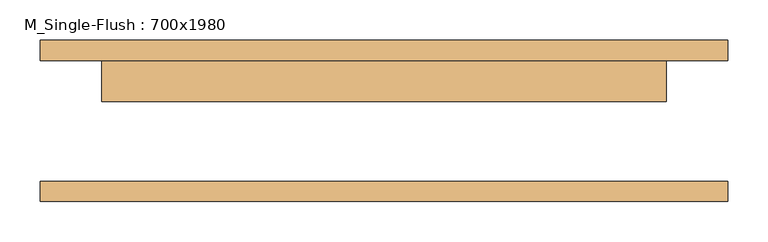
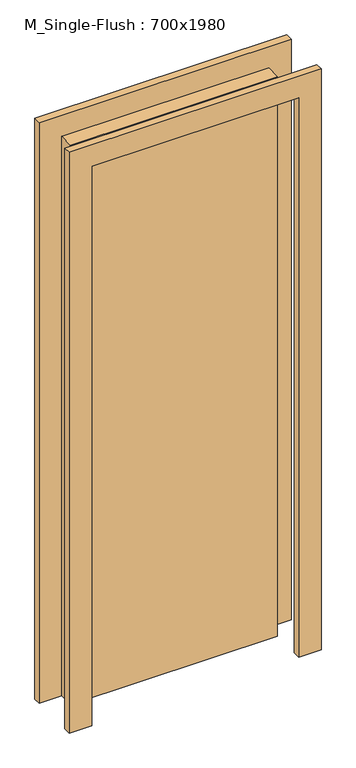
"""IFC4 building model written with IfcOpenShell, lengths in millimetres: door geometry, M_Single-Flush : 700x1980."""

from ifc_helpers import new_model, si_unit, frame, origin, origin_with_axes, place, context, project, spatial, polyline, outline, extrude, source, transform, mapped, element, save


def m_single_flush_700x1980_d4223ffa(model_context):
    return source(origin(), model_context, "Body", "SweptSolid", [
        extrude(outline(polyline([(2076.0, -426.0), (0.0, -426.0), (0.0, -350.0), (2000.0, -350.0), (2000.0, 350.0), (0.0, 350.0), (0.0, 426.0), (2076.0, 426.0), (2076.0, -426.0)])), frame((0.0, 75.0, 0.0), z_axis=(0.0, 1.0, 0.0), x_axis=(0.0, 0.0, 1.0)), (0.0, 0.0, 1.0), 25.0),
        extrude(outline(polyline([(2076.0, 426.0), (2076.0, -426.0), (0.0, -426.0), (0.0, -350.0), (2000.0, -350.0), (2000.0, 350.0), (0.0, 350.0), (0.0, 426.0), (2076.0, 426.0)])), frame((0.0, -100.0, 0.0), z_axis=(0.0, 1.0, 0.0), x_axis=(0.0, 0.0, 1.0)), (0.0, 0.0, 1.0), 25.0),
        extrude(outline(polyline([(350.0, 24.0), (-350.0, 24.0), (-350.0, 75.0), (350.0, 75.0), (350.0, 24.0)])), origin_with_axes(), (0.0, 0.0, 1.0), 2000.0),
    ])


if __name__ == "__main__":
    model = new_model("IFC4")
    model_context = context("Model", 3, world=origin())
    ifc_project = project(units=[si_unit("LENGTHUNIT", "METRE", prefix="MILLI")], contexts=[model_context])
    site = spatial("IfcSite", under=ifc_project)
    building = spatial("IfcBuilding", under=site)
    placement = place(None, origin())
    m_single_flush_700x1980_shape = m_single_flush_700x1980_d4223ffa(model_context)
    element("IfcDoor", 1, ObjectType="M_Single-Flush : 700x1980", at=placement, inside=building, context=model_context, shape_type="MappedRepresentation", body=[
        mapped(m_single_flush_700x1980_shape, transform((0.0, 0.0, 0.0), x_axis=(1.0, 0.0, 0.0), y_axis=(0.0, 1.0, 0.0), z_axis=(0.0, 0.0, 1.0))),
    ])
    save(model, "model.ifc")

# Revit data of these elements
# Type "M_Single-Flush : 700x1980"
#   Type Mark = "47"
#   Construction Type Id = "MDOOR"
#   Analytic Construction = "Metal"
#   Thickness = 51 mm
#   Thermal Resistance (R) = 0.270117 (m²·K)/W
#   Heat Transfer Coefficient (U) = 3.7021 W/(m²·K)
#   Height = 2000 mm
#   Trim Projection Ext = 25 mm
#   Trim Projection Int = 25 mm
#   Trim Width = 76 mm
#   Width = 700 mm
#   Define Thermal Properties by = 1
#   Door Material = Door - Panel
#   Frame Material = Door - Frame
#   Visual Light Transmittance = 0
#   Solar Heat Gain Coefficient = 0
#   Function = (empty or 0)
#   Wall Closure = (empty or 0)
# Element 1 (IfcDoor, "M_Single-Flush : 700x1980")
#   Materials on its faces: "Door - Frame", "Door - Panel"
# Materials
#   "Door - Panel": class "Wood", colour RGB 210 159 95, transparency 0, Cost = 0
#   "Door - Frame": colour RGB 118 70 51, transparency 0, Cost = 0
